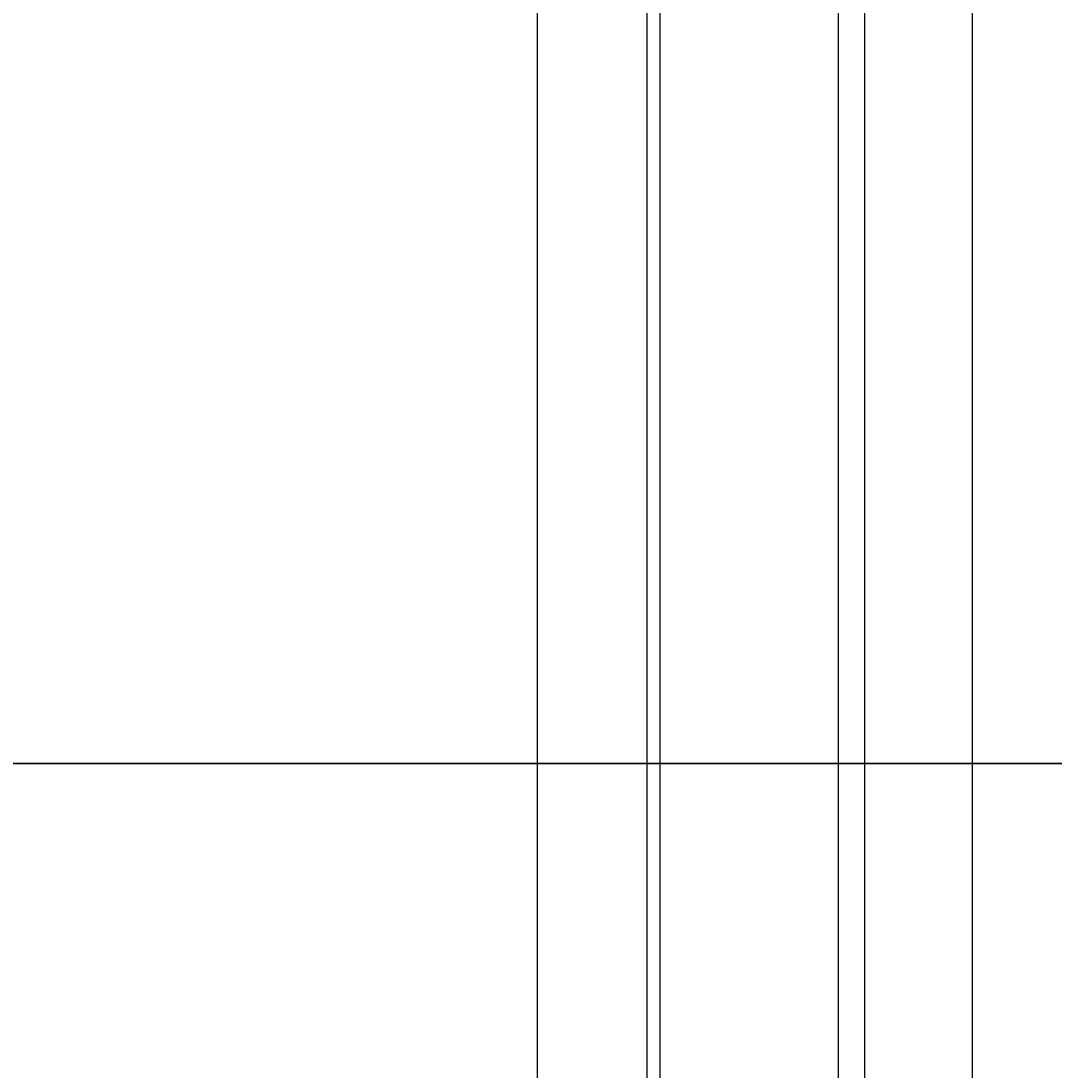
# Model space of a CAD drawing. Units: inches. Extents: x -6 to 289, y -8 to 323.
# Tile 83 of 107: x 150 to 173, y 252 to 276. Entities that reach past the tile are written whole.
import ezdxf

# ---------------------------------------------------------------- set-up
doc = ezdxf.new("R2010")
doc.units = ezdxf.units.IN
doc.header["$MEASUREMENT"] = 0
doc.layers.add('A-ANNO-DIMS', color=2, linetype='Continuous', lineweight=18)
doc.layers.add('A-ELEV', color=7, linetype='Continuous', lineweight=35)
doc.styles.get("Standard").update_dxf_attribs({"font": 'arial.ttf'})
doc.dimstyles.get("Standard").update_dxf_attribs({"dimtxt": 0.18, "dimasz": 0.18, "dimexe": 0.18, "dimexo": 0.0625, "dimgap": 0.09, "dimtad": 0, "dimtih": 1, "dimtoh": 1, "dimdec": 4, "dimzin": 0, "dimdsep": 46, "dimtxsty": 'Standard', "dimcen": 0.09, "dimadec": 0, "dimazin": 0, "dimtfac": 1, "dimtdec": 4, "dimtofl": 0, "dimtmove": 0, "dimatfit": 3, "dimfxl": 1, "dimtolj": 1, "dimtzin": 0, "dimarcsym": 0})

# ---------------------------------------------------------------- blocks, each defined once
blk = doc.blocks.new('*D11')
at = {"layer": 'A-ANNO-DIMS', "color": 0, "lineweight": -2, "transparency": 16777216}
for p, q in [((126.883, 226.717), (126.883, 322.969)), ((168.883, 226.717), (168.883, 322.969)), ((127.063, 322.789), (147.662, 322.789)), ((168.703, 322.789), (148.105, 322.789))]:
    blk.add_line(p, q, dxfattribs=at)
at = {"layer": 'A-ANNO-DIMS', "color": 0, "transparency": 16777216}
for points in [[(127.063, 322.819), (127.063, 322.759), (126.883, 322.789)], [(168.703, 322.819), (168.703, 322.759), (168.883, 322.789)]]:
    blk.add_solid(points, dxfattribs=at)
at = {"layer": 'Defpoints', "color": 0, "transparency": 16777216}
for p in [(168.883, 322.789), (126.883, 226.654), (168.883, 226.654)]:
    blk.add_point(p, dxfattribs=at)
at = {"layer": 'A-ANNO-DIMS', "color": 0, "transparency": 16777216, "insert": (147.883, 322.789), "char_height": 0.18, "attachment_point": 5}
blk.add_mtext('\\A1;42', dxfattribs=at)
blk = doc.blocks.new('*D12')
at = {"layer": 'A-ANNO-DIMS', "color": 0, "lineweight": -2, "transparency": 16777216}
for p, q in [((168.883, 226.717), (168.883, 322.969)), ((188.292, 226.951), (188.292, 322.969)), ((169.063, 322.789), (178.22, 322.789)), ((188.112, 322.789), (178.955, 322.789))]:
    blk.add_line(p, q, dxfattribs=at)
at = {"layer": 'A-ANNO-DIMS', "color": 0, "transparency": 16777216}
for points in [[(169.063, 322.819), (169.063, 322.759), (168.883, 322.789)], [(188.112, 322.819), (188.112, 322.759), (188.292, 322.789)]]:
    blk.add_solid(points, dxfattribs=at)
at = {"layer": 'Defpoints', "color": 0, "transparency": 16777216}
for p in [(188.292, 322.789), (188.292, 226.889), (168.883, 226.654)]:
    blk.add_point(p, dxfattribs=at)
at = {"layer": 'A-ANNO-DIMS', "color": 0, "transparency": 16777216, "insert": (178.588, 322.789), "char_height": 0.18, "attachment_point": 5}
blk.add_mtext('\\A1;19.41', dxfattribs=at)
blk = doc.blocks.new('*D27')
at = {"layer": 'A-ANNO-DIMS', "color": 0, "lineweight": -2, "transparency": 16777216}
for p, q in [((19.226, 307.289), (288.653, 307.289)), ((288.473, 307.109), (288.473, 277.471)), ((288.473, 247.469), (288.473, 277.107)), ((247.226, 247.289), (288.653, 247.289))]:
    blk.add_line(p, q, dxfattribs=at)
at = {"layer": 'A-ANNO-DIMS', "color": 0, "transparency": 16777216}
for points in [[(288.443, 307.109), (288.503, 307.109), (288.473, 307.289)], [(288.443, 247.469), (288.503, 247.469), (288.473, 247.289)]]:
    blk.add_solid(points, dxfattribs=at)
at = {"layer": 'Defpoints', "color": 0, "transparency": 16777216}
for p in [(19.164, 307.289), (288.473, 307.289), (247.164, 247.289)]:
    blk.add_point(p, dxfattribs=at)
at = {"layer": 'A-ANNO-DIMS', "color": 0, "transparency": 16777216, "insert": (288.473, 277.289), "char_height": 0.18, "attachment_point": 5}
blk.add_mtext('\\A1;60', dxfattribs=at)
blk = doc.blocks.new('*D76')
at = {"layer": 'A-ANNO-DIMS', "color": 0, "lineweight": -2, "transparency": 16777216}
for p, q in [((142.296, 51.148), (142.296, 322.969)), ((164.296, 51.148), (164.296, 322.969)), ((142.476, 322.789), (153.076, 322.789)), ((164.116, 322.789), (153.516, 322.789))]:
    blk.add_line(p, q, dxfattribs=at)
at = {"layer": 'A-ANNO-DIMS', "color": 0, "transparency": 16777216}
for points in [[(142.476, 322.819), (142.476, 322.759), (142.296, 322.789)], [(164.116, 322.819), (164.116, 322.759), (164.296, 322.789)]]:
    blk.add_solid(points, dxfattribs=at)
at = {"layer": 'Defpoints', "color": 0, "transparency": 16777216}
for p in [(164.296, 322.789), (142.296, 51.085), (164.296, 51.085)]:
    blk.add_point(p, dxfattribs=at)
at = {"layer": 'A-ANNO-DIMS', "color": 0, "transparency": 16777216, "insert": (153.296, 322.789), "char_height": 0.18, "attachment_point": 5}
blk.add_mtext('\\A1;22', dxfattribs=at)
blk = doc.blocks.new('*D77')
at = {"layer": 'A-ANNO-DIMS', "color": 0, "lineweight": -2, "transparency": 16777216}
for p, q in [((164.296, 51.148), (164.296, 322.969)), ((168.296, 51.148), (168.296, 322.969)), ((164.476, 322.789), (166.144, 322.789)), ((168.116, 322.789), (166.448, 322.789))]:
    blk.add_line(p, q, dxfattribs=at)
at = {"layer": 'A-ANNO-DIMS', "color": 0, "transparency": 16777216}
for points in [[(164.476, 322.819), (164.476, 322.759), (164.296, 322.789)], [(168.116, 322.819), (168.116, 322.759), (168.296, 322.789)]]:
    blk.add_solid(points, dxfattribs=at)
at = {"layer": 'Defpoints', "color": 0, "transparency": 16777216}
for p in [(168.296, 322.789), (164.296, 51.085), (168.296, 51.085)]:
    blk.add_point(p, dxfattribs=at)
at = {"layer": 'A-ANNO-DIMS', "color": 0, "transparency": 16777216, "insert": (166.296, 322.789), "char_height": 0.18, "attachment_point": 5}
blk.add_mtext('\\A1;4', dxfattribs=at)
blk = doc.blocks.new('*D78')
at = {"layer": 'A-ANNO-DIMS', "color": 0, "lineweight": -2, "transparency": 16777216}
for p, q in [((168.296, 51.148), (168.296, 322.969)), ((171.296, 51.148), (171.296, 322.969)), ((168.476, 322.789), (169.647, 322.789)), ((171.116, 322.789), (169.945, 322.789))]:
    blk.add_line(p, q, dxfattribs=at)
at = {"layer": 'A-ANNO-DIMS', "color": 0, "transparency": 16777216}
for points in [[(168.476, 322.819), (168.476, 322.759), (168.296, 322.789)], [(171.116, 322.819), (171.116, 322.759), (171.296, 322.789)]]:
    blk.add_solid(points, dxfattribs=at)
at = {"layer": 'Defpoints', "color": 0, "transparency": 16777216}
for p in [(171.296, 322.789), (168.296, 51.085), (171.296, 51.085)]:
    blk.add_point(p, dxfattribs=at)
at = {"layer": 'A-ANNO-DIMS', "color": 0, "transparency": 16777216, "insert": (169.796, 322.789), "char_height": 0.18, "attachment_point": 5}
blk.add_mtext('\\A1;3', dxfattribs=at)
blk = doc.blocks.new('*D79')
at = {"layer": 'A-ANNO-DIMS', "color": 0, "lineweight": -2, "transparency": 16777216}
for p, q in [((171.296, 118.033), (171.296, 322.969)), ((188.292, 116.842), (188.292, 322.969)), ((171.476, 322.789), (179.339, 322.789)), ((188.112, 322.789), (180.249, 322.789))]:
    blk.add_line(p, q, dxfattribs=at)
at = {"layer": 'A-ANNO-DIMS', "color": 0, "transparency": 16777216}
for points in [[(171.476, 322.819), (171.476, 322.759), (171.296, 322.789)], [(188.112, 322.819), (188.112, 322.759), (188.292, 322.789)]]:
    blk.add_solid(points, dxfattribs=at)
at = {"layer": 'Defpoints', "color": 0, "transparency": 16777216}
for p in [(188.292, 322.789), (171.296, 117.971), (188.292, 116.779)]:
    blk.add_point(p, dxfattribs=at)
at = {"layer": 'A-ANNO-DIMS', "color": 0, "transparency": 16777216, "insert": (179.794, 322.789), "char_height": 0.18, "attachment_point": 5}
blk.add_mtext('\\A1;16.996', dxfattribs=at)
blk = doc.blocks.new('*D94')
at = {"layer": 'A-ANNO-DIMS', "color": 0, "lineweight": -2, "transparency": 16777216}
for p, q in [((118.164, 159.411), (118.164, 322.969)), ((161.552, 159.411), (161.552, 322.969)), ((118.344, 322.789), (139.46, 322.789)), ((161.372, 322.789), (140.256, 322.789))]:
    blk.add_line(p, q, dxfattribs=at)
at = {"layer": 'A-ANNO-DIMS', "color": 0, "transparency": 16777216}
for points in [[(118.344, 322.819), (118.344, 322.759), (118.164, 322.789)], [(161.372, 322.819), (161.372, 322.759), (161.552, 322.789)]]:
    blk.add_solid(points, dxfattribs=at)
at = {"layer": 'Defpoints', "color": 0, "transparency": 16777216}
for p in [(161.552, 322.789), (118.164, 159.348), (161.552, 159.348)]:
    blk.add_point(p, dxfattribs=at)
at = {"layer": 'A-ANNO-DIMS', "color": 0, "transparency": 16777216, "insert": (139.858, 322.789), "char_height": 0.18, "attachment_point": 5}
blk.add_mtext('\\A1;43.39', dxfattribs=at)
blk = doc.blocks.new('*D95')
at = {"layer": 'A-ANNO-DIMS', "color": 0, "lineweight": -2, "transparency": 16777216}
for p, q in [((161.552, 159.411), (161.552, 322.969)), ((164.004, 159.411), (164.004, 322.969)), ((161.732, 322.789), (162.452, 322.789)), ((163.824, 322.789), (163.104, 322.789))]:
    blk.add_line(p, q, dxfattribs=at)
at = {"layer": 'A-ANNO-DIMS', "color": 0, "transparency": 16777216}
for points in [[(161.732, 322.819), (161.732, 322.759), (161.552, 322.789)], [(163.824, 322.819), (163.824, 322.759), (164.004, 322.789)]]:
    blk.add_solid(points, dxfattribs=at)
at = {"layer": 'Defpoints', "color": 0, "transparency": 16777216}
for p in [(164.004, 322.789), (161.552, 159.348), (164.004, 159.348)]:
    blk.add_point(p, dxfattribs=at)
at = {"layer": 'A-ANNO-DIMS', "color": 0, "transparency": 16777216, "insert": (162.778, 322.789), "char_height": 0.18, "attachment_point": 5}
blk.add_mtext('\\A1;2.45', dxfattribs=at)
blk = doc.blocks.new('*D96')
at = {"layer": 'A-ANNO-DIMS', "color": 0, "lineweight": -2, "transparency": 16777216}
for p, q in [((164.004, 159.411), (164.004, 322.969)), ((200.616, 159.411), (200.616, 322.969)), ((164.184, 322.789), (181.934, 322.789)), ((200.436, 322.789), (182.686, 322.789))]:
    blk.add_line(p, q, dxfattribs=at)
at = {"layer": 'A-ANNO-DIMS', "color": 0, "transparency": 16777216}
for points in [[(164.184, 322.819), (164.184, 322.759), (164.004, 322.789)], [(200.436, 322.819), (200.436, 322.759), (200.616, 322.789)]]:
    blk.add_solid(points, dxfattribs=at)
at = {"layer": 'Defpoints', "color": 0, "transparency": 16777216}
for p in [(200.616, 322.789), (164.004, 159.348), (200.616, 159.348)]:
    blk.add_point(p, dxfattribs=at)
at = {"layer": 'A-ANNO-DIMS', "color": 0, "transparency": 16777216, "insert": (182.31, 322.789), "char_height": 0.18, "attachment_point": 5}
blk.add_mtext('\\A1;36.61', dxfattribs=at)

msp = doc.modelspace()

# ---------------------------------------------------------------- linework, layer by layer
at = {"layer": 'A-ELEV'}
msp.add_line((115.1638, 259.2888), (271.1638, 259.2888), dxfattribs=at)

# ---------------------------------------------------------------- dimensions: what is measured, and where the dimension line sits
at = {"layer": 'A-ANNO-DIMS'}
for base, p1, p2, override, picture, middle in [((161.5522, 322.7888), (118.1638, 159.3484), (161.5522, 159.3484), {"dimdec": 2, "dimlfac": 1, "dimrnd": 0, "dimzin": 0, "dimdsep": 46, "dimlunit": 2}, '*D94', (139.858, 322.7888)), ((168.8835, 322.7888), (126.8835, 226.654), (168.8835, 226.654), {"dimdec": 0, "dimlfac": 1, "dimrnd": 0, "dimzin": 0, "dimdsep": 46, "dimlunit": 2}, '*D11', (147.8835, 322.7888)), ((164.296, 322.7888), (142.296, 51.0851), (164.296, 51.0851), {"dimdec": 0, "dimlfac": 1, "dimrnd": 0, "dimzin": 0, "dimdsep": 46, "dimlunit": 2}, '*D76', (153.296, 322.7888)), ((164.0039, 322.7888), (161.5522, 159.3484), (164.0039, 159.3484), {"dimdec": 2, "dimlfac": 1, "dimrnd": 0, "dimzin": 0, "dimdsep": 46, "dimlunit": 2}, '*D95', (162.7781, 322.7888)), ((200.6162, 322.7888), (164.0039, 159.3484), (200.6162, 159.3484), {"dimdec": 2, "dimlfac": 1, "dimrnd": 0, "dimzin": 0, "dimdsep": 46, "dimlunit": 2}, '*D96', (182.3101, 322.7888)), ((168.296, 322.7888), (164.296, 51.0851), (168.296, 51.0851), {"dimdec": 0, "dimlfac": 1, "dimrnd": 0, "dimzin": 0, "dimdsep": 46, "dimlunit": 2}, '*D77', (166.296, 322.7888)), ((171.296, 322.7888), (168.296, 51.0851), (171.296, 51.0851), {"dimdec": 0, "dimlfac": 1, "dimrnd": 0, "dimzin": 0, "dimdsep": 46, "dimlunit": 2}, '*D78', (169.796, 322.7888)), ((188.2918, 322.7888), (168.8835, 226.654), (188.2918, 226.8887), {"dimdec": 2, "dimlfac": 1, "dimrnd": 0, "dimzin": 0, "dimdsep": 46, "dimlunit": 2}, '*D12', (178.5876, 322.7888)), ((188.2918, 322.7888), (171.296, 117.9706), (188.2918, 116.7795), {"dimdec": 3, "dimlfac": 1, "dimrnd": 0, "dimzin": 0, "dimdsep": 46, "dimlunit": 2}, '*D79', (179.7939, 322.7888))]:
    dim = msp.add_linear_dim(base=base, p1=p1, p2=p2, dimstyle='Standard', override=override, dxfattribs=at)
    dim.commit()
    dim.dimension.update_dxf_attribs({"geometry": picture, "text_midpoint": middle})
dim = msp.add_linear_dim(base=(288.4733, 307.2888), p1=(247.1638, 247.2888), p2=(19.1638, 307.2888), angle=90, dimstyle='Standard', override={"dimdec": 0, "dimlfac": 1, "dimrnd": 0, "dimzin": 0, "dimdsep": 46, "dimlunit": 2}, dxfattribs=at)
dim.commit()
dim.dimension.update_dxf_attribs({"geometry": '*D27', "text_midpoint": (288.4733, 277.2888)})

doc.saveas('drawing.dxf')
